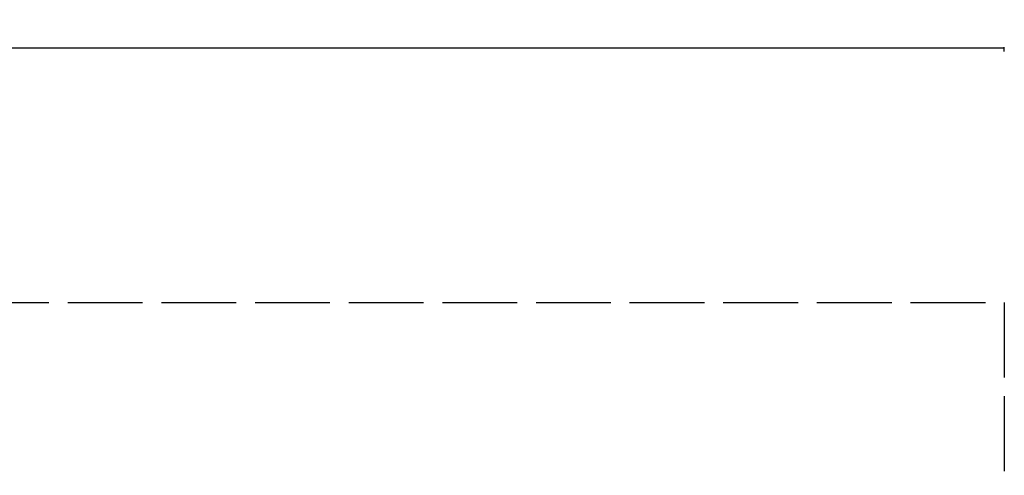
# Model space of a CAD drawing. Units: inches. Extents: x 1316 to 1777, y 813 to 1650.
# Tile 22 of 22: x 1567 to 1724, y 1576 to 1650. Entities that reach past the tile are written whole.
import ezdxf

# ---------------------------------------------------------------- set-up
doc = ezdxf.new("R2010")
doc.units = ezdxf.units.IN
doc.header["$MEASUREMENT"] = 0
doc.linetypes.add('ACAD_ISO02W100', pattern=[15, 12, -3])
doc.layers.add('A-ANNO-DIMS', color=2, linetype='Continuous', lineweight=18)
doc.layers.add('C-PROP', color=8, linetype='ACAD_ISO02W100', lineweight=25)
doc.styles.get("Standard").update_dxf_attribs({"font": 'arial.ttf'})
doc.dimstyles.get("Standard").update_dxf_attribs({"dimtxt": 7, "dimasz": 0.18, "dimexe": 0.18, "dimexo": 0.0625, "dimgap": 0.09, "dimtad": 0, "dimtih": 1, "dimtoh": 1, "dimzin": 0, "dimdsep": 46, "dimlunit": 3, "dimtxsty": 'Standard', "dimcen": 0.09, "dimadec": 0, "dimazin": 0, "dimtfac": 1, "dimtofl": 0, "dimtmove": 0, "dimatfit": 3, "dimfxl": 1, "dimtolj": 1, "dimtzin": 0, "dimarcsym": 0})

# ---------------------------------------------------------------- blocks, each defined once
blk = doc.blocks.new('*D22')
at = {"layer": 'A-ANNO-DIMS', "color": 0, "lineweight": -2, "transparency": 16777216}
for p, q in [((1364.4, 1644.46), (1364.4, 1645.13)), ((1364.58, 1644.95), (1532.29, 1644.95)), ((1724.22, 1644.95), (1556.51, 1644.95)), ((1724.4, 1644.46), (1724.4, 1645.13))]:
    blk.add_line(p, q, dxfattribs=at)
at = {"layer": 'A-ANNO-DIMS', "color": 0, "transparency": 16777216}
for points in [[(1364.58, 1644.98), (1364.58, 1644.92), (1364.4, 1644.95)], [(1724.22, 1644.98), (1724.22, 1644.92), (1724.4, 1644.95)]]:
    blk.add_solid(points, dxfattribs=at)
at = {"layer": 'Defpoints', "color": 0, "transparency": 16777216}
for p in [(1724.4, 1644.95), (1364.4, 1644.4), (1724.4, 1644.4)]:
    blk.add_point(p, dxfattribs=at)
at = {"layer": 'A-ANNO-DIMS', "color": 0, "transparency": 16777216, "insert": (1544.4, 1644.95), "char_height": 7, "attachment_point": 5}
blk.add_mtext('\\A1;30\'-0"', dxfattribs=at)

msp = doc.modelspace()

# ---------------------------------------------------------------- linework, layer by layer
at = {"layer": 'C-PROP'}
for p, q in [((1364.399, 1604.173), (1724.399, 1604.173)), ((1724.399, 1604.173), (1724.399, 1040.173))]:
    msp.add_line(p, q, dxfattribs=at)

# ---------------------------------------------------------------- dimensions: what is measured, and where the dimension line sits
at = {"layer": 'A-ANNO-DIMS'}
dim = msp.add_linear_dim(base=(1724.399, 1644.949), p1=(1364.399, 1644.396), p2=(1724.399, 1644.396), text='30\'-0"', dimstyle='Standard', override={"dimclrd": 0, "dimclre": 0, "dimclrt": 0}, dxfattribs=at)
dim.commit()
dim.dimension.update_dxf_attribs({"geometry": '*D22', "text_midpoint": (1544.399, 1644.949)})

doc.saveas('drawing.dxf')
